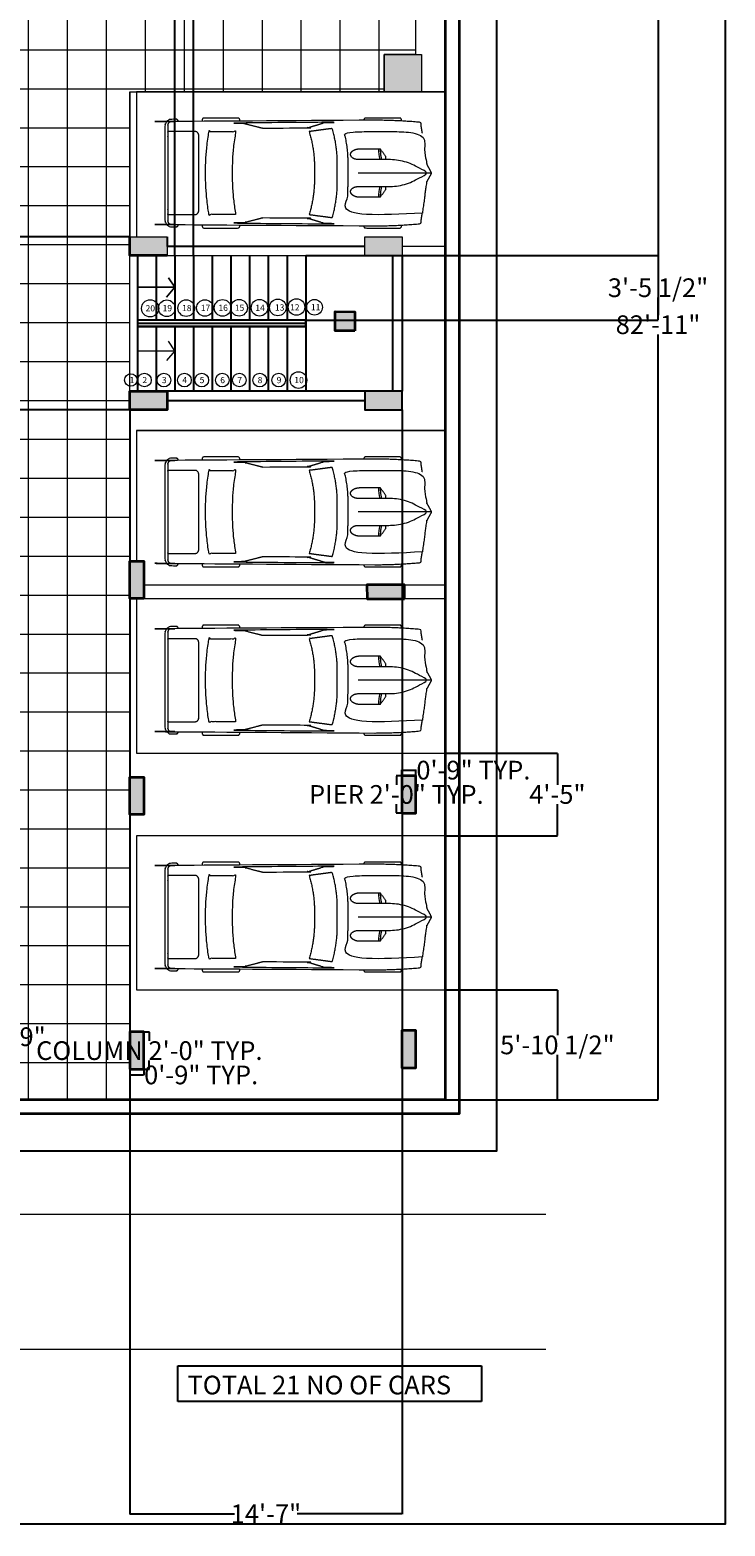
# Model space of a CAD drawing. Units: inches. Extents: x 48986 to 50522, y 132527 to 134098.
# Tile 3 of 4: x 50076 to 50522, y 132527 to 133488. Entities that reach past the tile are written whole.
import ezdxf

# ---------------------------------------------------------------- set-up
doc = ezdxf.new("R2010")
doc.units = ezdxf.units.IN
doc.header["$MEASUREMENT"] = 0
for name, color, linetype, lineweight in [('A-ANNO-DIMS', 2, 'Continuous', 18), ('A-ANNO-SYMB', 50, 'Continuous', 13), ('A-ANNO-TEXT', 7, 'Continuous', 18), ('A-ANNO-TTLB', 7, 'Continuous', 25), ('A-COLS-PATT', 215, 'Continuous', 13), ('A-EQPM-VEHC', 8, 'Continuous', 13), ('A-FLOR-PATT', 94, 'Continuous', 9), ('A-FLOR-PKNG', 140, 'Continuous', 18), ('C-PROP', 160, 'Continuous', 25), ('C-ROAD', 7, 'Continuous', 18), ('COLUMNS', 211, 'Continuous', 35), ('STAIRS', 10, 'Continuous', 25), ('WALLS', 140, 'Continuous', 35)]:
    doc.layers.add(name, color=color, linetype=linetype, lineweight=lineweight)
doc.styles.get("Standard").update_dxf_attribs({"font": 'arial.ttf'})
doc.dimstyles.get("Standard").update_dxf_attribs({"dimtxt": 12, "dimasz": 0.18, "dimexe": 0.18, "dimexo": 0.0625, "dimgap": 0.09, "dimtad": 0, "dimtih": 1, "dimtoh": 1, "dimdec": 1, "dimzin": 0, "dimdsep": 46, "dimlunit": 3, "dimtxsty": 'Standard', "dimcen": 0.09, "dimadec": 0, "dimazin": 0, "dimtfac": 1, "dimtdec": 1, "dimtofl": 0, "dimtmove": 0, "dimatfit": 3, "dimfxl": 1, "dimtolj": 1, "dimtzin": 0, "dimarcsym": 0})

# ---------------------------------------------------------------- blocks, each defined once
blk = doc.blocks.new('CAR-SEDAN-PLAN')
for p, q in [((35.28, 177.53), (35.28, 130.65)), ((25.73, 8.37), (44.83, 8.37))]:
    blk.add_line(p, q)
for centre, major_axis, start_param, end_param in [((19.85, 164.65), (-24.87, 0), 1.564964, 1.848039), ((50.71, 164.65), (24.87, 0), 4.435146, 4.718221)]:
    blk.add_ellipse(centre, major_axis=major_axis, ratio=0.842304, start_param=start_param, end_param=end_param)
for points, weights, knots in [([(60.93, 171.77), (56.4, 172.48), (51.85, 173.06), (46.33, 173.7), (40.84, 174.57), (38.25, 176), (35.65, 177.44), (35.28, 177.64), (34.91, 177.44), (32.32, 176), (29.72, 174.57), (24.24, 173.7), (18.71, 173.06), (14.16, 172.48), (9.64, 171.77), (7.88, 146.82), (9.23, 121.85), (17.23, 123.66), (25.51, 124.08), (35.28, 124.08), (45.06, 124.08), (53.33, 123.66), (61.34, 121.85), (62.69, 146.82), (60.93, 171.77)], [1, 0.999861960732, 1, 0.999699858145, 1, 1, 1, 0.835952709181, 1, 1, 1, 0.999699858145, 1, 0.999861960732, 1, 0.998625728423, 1, 0.994860280211, 1, 1, 1, 0.994860280211, 1, 0.998625728423, 1], [0, 0, 0, 0.033232, 0.033232, 0.082234, 0.082234, 1.082234, 1.082234, 2.244094, 2.244094, 3.244094, 3.244094, 3.293097, 3.293097, 3.326328, 3.326328, 3.431193, 3.431193, 3.634055, 3.634055, 4.634055, 4.634055, 4.836917, 4.836917, 4.941783, 4.941783, 4.941783]), ([(43.91, 145.56), (47.31, 144.74), (50.86, 144.76), (50.86, 138.04), (50.86, 131.32), (50.59, 126.02), (47.38, 125.71), (44.17, 125.4), (43.91, 130.65), (43.91, 140.58), (43.91, 150.52), (43.91, 163.57), (35.28, 174.41), (26.66, 163.57), (26.66, 150.52), (26.66, 140.58), (26.66, 130.65), (26.39, 125.4), (23.18, 125.71), (19.97, 126.02), (19.71, 131.32), (19.71, 138.04), (19.71, 144.76), (23.25, 144.74), (26.66, 145.56)], [1, 0.990000279832, 1, 1, 1, 0.735618766318, 1, 0.735618766318, 1, 1, 1, 0.956755789522, 1, 0.956755789522, 1, 1, 1, 0.735618766318, 1, 0.735618766318, 1, 1, 1, 0.990000279832, 1], [0, 0, 0, 0.283075, 0.283075, 1.283075, 1.283075, 2.771508, 2.771508, 4.259942, 4.259942, 5.259942, 5.259942, 5.85026, 5.85026, 6.440579, 6.440579, 7.440579, 7.440579, 8.929012, 8.929012, 10.417446, 10.417446, 11.417446, 11.417446, 11.700521, 11.700521, 11.700521]), ([(9.64, 171.77), (6.18, 171.25), (2.75, 170.65), (1.43, 155.99), (1.38, 141.3)], [1, 0.999923835344, 1, 0.999337806115, 1], [0, 0, 0, 0.02468451, 0.02468451, 0.0974728, 0.0974728, 0.0974728]), ([(69.18, 141.3), (69.13, 155.99), (67.82, 170.65), (64.38, 171.25), (60.93, 171.77)], [1, 0.999337806115, 1, 0.999923835344, 1], [0, 0, 0, 0.07278829, 0.07278829, 0.0974728, 0.0974728, 0.0974728]), ([(1.87, 158.39), (1.61, 158.39), (1.35, 158.39), (0.79, 158.39), (0.4, 158.06), (0, 157.72), (0, 157.26), (0, 146.28), (0, 135.3), (0, 134.83), (0.4, 134.5), (0.79, 134.17), (1.35, 134.17), (1.35, 134.17), (1.36, 134.17)], [1, 1, 1, 0.923879532511, 1, 0.923879532511, 1, 1, 1, 0.923879532511, 1, 0.923879532511, 1, 1, 1], [0, 0, 0, 1, 1, 1.785398, 1.785398, 2.570796, 2.570796, 3.570796, 3.570796, 4.356194, 4.356194, 5.141593, 5.141593, 6.141593, 6.141593, 6.141593]), ([(69.2, 134.17), (69.21, 134.17), (69.22, 134.17), (69.77, 134.17), (70.17, 134.5), (70.56, 134.83), (70.56, 135.3), (70.56, 146.28), (70.56, 157.26), (70.56, 157.72), (70.17, 158.06), (69.77, 158.39), (69.22, 158.39), (68.96, 158.39), (68.7, 158.39)], [1, 1, 1, 0.923879532511, 1, 0.923879532511, 1, 1, 1, 0.923879532511, 1, 0.923879532511, 1, 1, 1], [0, 0, 0, 1, 1, 1.785398, 1.785398, 2.570796, 2.570796, 3.570796, 3.570796, 4.356194, 4.356194, 5.141593, 5.141593, 6.141593, 6.141593, 6.141593]), ([(26.66, 148.39), (25.91, 148.39), (25.16, 148.39), (24.92, 148.39), (24.74, 148.26), (22.22, 146.51), (19.71, 144.76)], [1, 1, 1, 0.940892222322, 1, 1, 1], [0, 0, 0, 1, 1, 1.691083, 1.691083, 2.691083, 2.691083, 2.691083]), ([(50.86, 144.76), (48.34, 146.51), (45.83, 148.26), (45.64, 148.39), (45.4, 148.39), (44.65, 148.39), (43.91, 148.39)], [1, 1, 1, 0.940892222322, 1, 1, 1], [0, 0, 0, 1, 1, 1.691083, 1.691083, 2.691083, 2.691083, 2.691083]), ([(1.38, 141.68), (1.17, 76.13), (2.21, 10.6), (2.24, 8.37), (4.89, 8.37), (35.28, 8.37), (65.67, 8.37), (68.32, 8.37), (68.36, 10.6), (69.4, 76.13), (69.18, 141.68)], [1, 0.999967219517, 1, 0.711827418646, 1, 1, 1, 0.711827418646, 1, 0.999967219517, 1], [0, 0, 0, 0.016194, 0.016194, 1.573593, 1.573593, 2.573593, 2.573593, 4.130993, 4.130993, 4.147187, 4.147187, 4.147187]), ([(6.45, 69.32), (4.72, 62.5), (2.98, 55.69), (2.73, 82.7), (2.7, 109.71), (4.53, 103.71), (6.37, 97.71), (6.33, 83.51), (6.45, 69.32)], [1, 1, 1, 0.999994429546, 1, 1, 1, 0.999987377106, 1], [0, 0, 0, 1, 1, 1.006676, 1.006676, 2.006676, 2.006676, 2.016725, 2.016725, 2.016725]), ([(61.91, 99.15), (52.72, 101.89), (42.99, 102.47), (35.28, 102.47), (27.57, 102.47), (17.85, 101.89), (8.66, 99.15), (7.66, 106.57), (6.67, 114), (15.95, 116.64), (25.73, 117.16), (35.28, 117.16), (44.83, 117.16), (54.61, 116.64), (63.89, 114), (62.9, 106.57), (61.91, 99.15)], [1, 0.991000078903, 1, 1, 1, 0.991000078903, 1, 1, 1, 0.991394232237, 1, 1, 1, 0.991394232237, 1, 1, 1], [0, 0, 0, 0.268529, 0.268529, 1.268529, 1.268529, 1.537057, 1.537057, 2.537057, 2.537057, 2.799631, 2.799631, 3.799631, 3.799631, 4.062205, 4.062205, 5.062205, 5.062205, 5.062205]), ([(64.11, 69.32), (64.24, 83.51), (64.2, 97.71), (66.03, 103.71), (67.87, 109.71), (67.83, 82.7), (67.58, 55.69), (65.85, 62.5), (64.11, 69.32)], [1, 0.999987377106, 1, 1, 1, 0.999994429546, 1, 1, 1], [0, 0, 0, 0.010049, 0.010049, 1.010049, 1.010049, 1.016725, 1.016725, 2.016725, 2.016725, 2.016725]), ([(1.65, 54.65), (1.5, 54.65), (1.35, 54.65), (0, 54.65), (0, 53.52), (0, 42.54), (0, 31.57), (0, 30.44), (1.35, 30.44), (1.63, 30.44), (1.92, 30.44)], [1, 1, 1, 0.707106781187, 1, 1, 1, 0.707106781187, 1, 1, 1], [0, 0, 0, 1, 1, 2.570796, 2.570796, 3.570796, 3.570796, 5.141593, 5.141593, 6.141593, 6.141593, 6.141593]), ([(61.91, 51.96), (35.28, 47.39), (8.66, 51.96), (8.66, 43.42), (8.66, 34.88), (35.28, 30.31), (61.91, 34.88), (61.91, 43.42), (61.91, 51.96)], [1, 0.979868494456, 1, 1, 1, 0.979868494456, 1, 1, 1], [0, 0, 0, 0.401989, 0.401989, 1.401989, 1.401989, 1.803978, 1.803978, 2.803978, 2.803978, 2.803978]), ([(68.64, 30.44), (68.93, 30.44), (69.22, 30.44), (69.77, 30.44), (70.17, 30.77), (70.56, 31.1), (70.56, 31.57), (70.56, 42.54), (70.56, 53.52), (70.56, 53.99), (70.17, 54.32), (69.77, 54.65), (69.22, 54.65), (69.07, 54.65), (68.91, 54.65)], [1, 1, 1, 0.923879532511, 1, 0.923879532511, 1, 1, 1, 0.923879532511, 1, 0.923879532511, 1, 1, 1], [0, 0, 0, 1, 1, 1.785398, 1.785398, 2.570796, 2.570796, 3.570796, 3.570796, 4.356194, 4.356194, 5.141593, 5.141593, 6.141593, 6.141593, 6.141593]), ([(61.91, 8.37), (61.91, 17.2), (61.91, 26.03), (61.91, 28.29), (59.22, 28.29), (35.28, 28.29), (11.34, 28.29), (8.66, 28.29), (8.66, 26.03), (8.66, 17.2), (8.66, 8.37)], [1, 1, 1, 0.707106781187, 1, 1, 1, 0.707106781187, 1, 1, 1], [0, 0, 0, 1, 1, 2.570796, 2.570796, 3.570796, 3.570796, 5.141593, 5.141593, 6.141593, 6.141593, 6.141593]), ([(2.14, 15.28), (0.74, 14.89), (0.76, 13.65), (0.78, 12.11), (0.81, 10.58), (0.87, 6.62), (5.56, 6.62), (35.28, 6.62), (65, 6.62), (69.7, 6.62), (69.76, 10.58), (69.78, 12.11), (69.81, 13.65), (69.83, 14.89), (68.43, 15.28)], [1, 0.807168985933, 1, 0.999999981995, 1, 0.711827418646, 1, 1, 1, 0.711827418646, 1, 0.999999981995, 1, 0.807168985459, 1], [0, 0, 0, 1.262912, 1.262912, 1.263291, 1.263291, 2.82069, 2.82069, 3.82069, 3.82069, 5.37809, 5.37809, 5.378469, 5.378469, 6.641381, 6.641381, 6.641381])]:
    blk.add_rational_spline(points, weights, degree=2, knots=knots)
blk = doc.blocks.new('PARKING-STALL-99X198')
blk.add_lwpolyline([(198, 0), (198, 99), (0, 99), (0, 0)], close=True)
blk = doc.blocks.new('PIER-9X24-PERIM')
blk.add_lwpolyline([(9, 12), (9, 24), (0, 24), (0, 0), (9, 0), (9, 24)])
blk = doc.blocks.new('COL-9X24')
blk.add_lwpolyline([(0, 0), (9, 0), (9, 24), (0, 24)], close=True)
blk = doc.blocks.new('*D19')
at = {"layer": 'A-ANNO-DIMS', "color": 0, "lineweight": -2, "transparency": 16777216}
for p, q in [((50314.54, 133009.06), (50310.82, 133009.06)), ((50311, 133008.88), (50311, 133003.27)), ((50311, 132985.24), (50311, 132990.84)), ((50314.54, 132985.06), (50310.82, 132985.06))]:
    blk.add_line(p, q, dxfattribs=at)
at = {"layer": 'A-ANNO-DIMS', "color": 0, "transparency": 16777216}
for points in [[(50310.97, 133008.88), (50311.03, 133008.88), (50311, 133009.06)], [(50310.97, 132985.24), (50311.03, 132985.24), (50311, 132985.06)]]:
    blk.add_solid(points, dxfattribs=at)
at = {"layer": 'Defpoints', "color": 0, "transparency": 16777216}
for p in [(50311, 133009.06), (50314.6, 133009.06), (50314.6, 132985.06)]:
    blk.add_point(p, dxfattribs=at)
at = {"layer": 'A-ANNO-DIMS', "color": 0, "transparency": 16777216, "insert": (50311, 132997.06), "char_height": 12, "attachment_point": 5}
blk.add_mtext('\\A1;PIER 2\'-0" TYP.', dxfattribs=at)
blk = doc.blocks.new('*D20')
at = {"layer": 'A-ANNO-DIMS', "color": 0, "lineweight": -2, "transparency": 16777216}
for p, q in [((50314.6, 133009.12), (50314.6, 133012.84)), ((50314.78, 133012.66), (50323.42, 133012.66)), ((50323.6, 133009.12), (50323.6, 133012.84)), ((50323.6, 133012.66), (50323.78, 133012.66))]:
    blk.add_line(p, q, dxfattribs=at)
at = {"layer": 'A-ANNO-DIMS', "color": 0, "transparency": 16777216}
for points in [[(50314.78, 133012.69), (50314.78, 133012.63), (50314.6, 133012.66)], [(50323.42, 133012.69), (50323.42, 133012.63), (50323.6, 133012.66)]]:
    blk.add_solid(points, dxfattribs=at)
at = {"layer": 'Defpoints', "color": 0, "transparency": 16777216}
for p in [(50323.6, 133012.66), (50314.6, 133009.06), (50323.6, 133009.06)]:
    blk.add_point(p, dxfattribs=at)
at = {"layer": 'A-ANNO-DIMS', "color": 0, "transparency": 16777216, "insert": (50360.44, 133012.66), "char_height": 12, "attachment_point": 5}
blk.add_mtext('\\A1;0\'-9" TYP.', dxfattribs=at)
blk = doc.blocks.new('*D23')
at = {"layer": 'A-ANNO-DIMS', "color": 0, "lineweight": -2, "transparency": 16777216}
for p, q in [((50148.94, 132844.64), (50152.66, 132844.64)), ((50152.48, 132844.46), (50152.48, 132838.94)), ((50148.94, 132820.64), (50152.66, 132820.64)), ((50152.48, 132820.82), (50152.48, 132826.34))]:
    blk.add_line(p, q, dxfattribs=at)
at = {"layer": 'A-ANNO-DIMS', "color": 0, "transparency": 16777216}
for points in [[(50152.45, 132844.46), (50152.51, 132844.46), (50152.48, 132844.64)], [(50152.45, 132820.82), (50152.51, 132820.82), (50152.48, 132820.64)]]:
    blk.add_solid(points, dxfattribs=at)
at = {"layer": 'Defpoints', "color": 0, "transparency": 16777216}
for p in [(50148.88, 132844.64), (50152.48, 132844.64), (50148.88, 132820.64)]:
    blk.add_point(p, dxfattribs=at)
at = {"layer": 'A-ANNO-DIMS', "color": 0, "transparency": 16777216, "insert": (50152.48, 132832.64), "char_height": 12, "attachment_point": 5}
blk.add_mtext('\\A1;COLUMN 2\'-0" TYP.', dxfattribs=at)
blk = doc.blocks.new('*D24')
at = {"layer": 'A-ANNO-DIMS', "color": 0, "lineweight": -2, "transparency": 16777216}
for p, q in [((50139.88, 132820.58), (50139.88, 132816.86)), ((50140.06, 132817.04), (50148.7, 132817.04)), ((50148.88, 132820.58), (50148.88, 132816.86)), ((50148.88, 132817.04), (50149.06, 132817.04))]:
    blk.add_line(p, q, dxfattribs=at)
at = {"layer": 'A-ANNO-DIMS', "color": 0, "transparency": 16777216}
for points in [[(50140.06, 132817.07), (50140.06, 132817.01), (50139.88, 132817.04)], [(50148.7, 132817.07), (50148.7, 132817.01), (50148.88, 132817.04)]]:
    blk.add_solid(points, dxfattribs=at)
at = {"layer": 'Defpoints', "color": 0, "transparency": 16777216}
for p in [(50139.88, 132820.64), (50148.88, 132820.64), (50148.88, 132817.04)]:
    blk.add_point(p, dxfattribs=at)
at = {"layer": 'A-ANNO-DIMS', "color": 0, "transparency": 16777216, "insert": (50185.73, 132817.04), "char_height": 12, "attachment_point": 5}
blk.add_mtext('\\A1;0\'-9" TYP.', dxfattribs=at)
blk = doc.blocks.new('*D26')
at = {"layer": 'A-ANNO-DIMS', "color": 0, "lineweight": -2, "transparency": 16777216}
for p, q in [((50342.35, 133796.06), (50479.12, 133796.06)), ((50478.94, 133795.88), (50478.94, 133304.77)), ((50478.94, 132801.24), (50478.94, 133292.34)), ((50342.35, 132801.06), (50479.12, 132801.06))]:
    blk.add_line(p, q, dxfattribs=at)
at = {"layer": 'A-ANNO-DIMS', "color": 0, "transparency": 16777216}
for points in [[(50478.91, 133795.88), (50478.97, 133795.88), (50478.94, 133796.06)], [(50478.91, 132801.24), (50478.97, 132801.24), (50478.94, 132801.06)]]:
    blk.add_solid(points, dxfattribs=at)
at = {"layer": 'Defpoints', "color": 0, "transparency": 16777216}
for p in [(50342.29, 133796.06), (50342.29, 132801.06), (50478.94, 132801.06)]:
    blk.add_point(p, dxfattribs=at)
at = {"layer": 'A-ANNO-DIMS', "color": 0, "transparency": 16777216, "insert": (50478.94, 133298.56), "char_height": 12, "attachment_point": 5}
blk.add_mtext('\\A1;82\'-11"', dxfattribs=at)
blk = doc.blocks.new('*D29')
at = {"layer": 'A-ANNO-DIMS', "color": 0, "lineweight": -2, "transparency": 16777216}
for p, q in [((50342.35, 132871.56), (50414.52, 132871.56)), ((50414.34, 132871.38), (50414.34, 132842.6)), ((50414.34, 132801.24), (50414.34, 132830.01)), ((50342.35, 132801.06), (50414.52, 132801.06))]:
    blk.add_line(p, q, dxfattribs=at)
at = {"layer": 'A-ANNO-DIMS', "color": 0, "transparency": 16777216}
for points in [[(50414.31, 132871.38), (50414.37, 132871.38), (50414.34, 132871.56)], [(50414.31, 132801.24), (50414.37, 132801.24), (50414.34, 132801.06)]]:
    blk.add_solid(points, dxfattribs=at)
at = {"layer": 'Defpoints', "color": 0, "transparency": 16777216}
for p in [(50342.29, 132871.56), (50342.29, 132801.06), (50414.34, 132801.06)]:
    blk.add_point(p, dxfattribs=at)
at = {"layer": 'A-ANNO-DIMS', "color": 0, "transparency": 16777216, "insert": (50414.34, 132836.31), "char_height": 12, "attachment_point": 5}
blk.add_mtext('\\A1;5\'-10 1/2"', dxfattribs=at)
blk = doc.blocks.new('*D30')
at = {"layer": 'A-ANNO-DIMS', "color": 0, "lineweight": -2, "transparency": 16777216}
for p, q in [((50139.82, 133355.06), (49029.36, 133355.06)), ((49029.54, 133354.88), (49029.54, 133305.73)), ((49029.54, 133244.15), (49029.54, 133293.29)), ((50139.82, 133243.97), (49029.36, 133243.97))]:
    blk.add_line(p, q, dxfattribs=at)
at = {"layer": 'A-ANNO-DIMS', "color": 0, "transparency": 16777216}
for points in [[(49029.51, 133354.88), (49029.57, 133354.88), (49029.54, 133355.06)], [(49029.51, 133244.15), (49029.57, 133244.15), (49029.54, 133243.97)]]:
    blk.add_solid(points, dxfattribs=at)
at = {"layer": 'Defpoints', "color": 0, "transparency": 16777216}
for p in [(49029.54, 133355.06), (50139.88, 133355.06), (50139.88, 133243.97)]:
    blk.add_point(p, dxfattribs=at)
at = {"layer": 'A-ANNO-DIMS', "color": 0, "transparency": 16777216, "insert": (49029.54, 133299.51), "char_height": 12, "attachment_point": 5}
blk.add_mtext('\\A1;9\'-3"', dxfattribs=at)
blk = doc.blocks.new('*D31')
at = {"layer": 'A-ANNO-DIMS', "color": 0, "lineweight": -2, "transparency": 16777216}
for p, q in [((50139.88, 133243.91), (50139.88, 132535.17)), ((50314.72, 133243.91), (50314.72, 132535.17)), ((50140.06, 132535.35), (50207.17, 132535.35)), ((50314.54, 132535.35), (50247.44, 132535.35))]:
    blk.add_line(p, q, dxfattribs=at)
at = {"layer": 'A-ANNO-DIMS', "color": 0, "transparency": 16777216}
for points in [[(50140.06, 132535.38), (50140.06, 132535.32), (50139.88, 132535.35)], [(50314.54, 132535.38), (50314.54, 132535.32), (50314.72, 132535.35)]]:
    blk.add_solid(points, dxfattribs=at)
at = {"layer": 'Defpoints', "color": 0, "transparency": 16777216}
for p in [(50139.88, 133243.97), (50314.72, 133243.97), (50314.72, 132535.35)]:
    blk.add_point(p, dxfattribs=at)
at = {"layer": 'A-ANNO-DIMS', "color": 0, "transparency": 16777216, "insert": (50227.3, 132535.35), "char_height": 12, "attachment_point": 5}
blk.add_mtext('\\A1;14\'-7"', dxfattribs=at)
blk = doc.blocks.new('*D37')
at = {"layer": 'A-ANNO-DIMS', "color": 0, "lineweight": -2, "transparency": 16777216}
for p, q in [((50342.35, 133023.56), (50414.52, 133023.56)), ((50414.34, 133023.38), (50414.34, 133003.25)), ((50414.34, 132970.74), (50414.34, 132990.86)), ((50342.35, 132970.56), (50414.52, 132970.56))]:
    blk.add_line(p, q, dxfattribs=at)
at = {"layer": 'A-ANNO-DIMS', "color": 0, "transparency": 16777216}
for points in [[(50414.31, 133023.38), (50414.37, 133023.38), (50414.34, 133023.56)], [(50414.31, 132970.74), (50414.37, 132970.74), (50414.34, 132970.56)]]:
    blk.add_solid(points, dxfattribs=at)
at = {"layer": 'Defpoints', "color": 0, "transparency": 16777216}
for p in [(50342.29, 133023.56), (50342.29, 132970.56), (50414.34, 132970.56)]:
    blk.add_point(p, dxfattribs=at)
at = {"layer": 'A-ANNO-DIMS', "color": 0, "transparency": 16777216, "insert": (50414.34, 132997.06), "char_height": 12, "attachment_point": 5}
blk.add_mtext('\\A1;4\'-5"', dxfattribs=at)
blk = doc.blocks.new('*D38')
at = {"layer": 'A-ANNO-DIMS', "color": 0, "lineweight": -2, "transparency": 16777216}
for p, q in [((49995.94, 132882.05), (50068.11, 132882.05)), ((50067.93, 132881.87), (50067.93, 132847.77)), ((50067.93, 132801.24), (50067.93, 132835.33)), ((49995.94, 132801.06), (50068.11, 132801.06))]:
    blk.add_line(p, q, dxfattribs=at)
at = {"layer": 'A-ANNO-DIMS', "color": 0, "transparency": 16777216}
for points in [[(50067.9, 132881.87), (50067.96, 132881.87), (50067.93, 132882.05)], [(50067.9, 132801.24), (50067.96, 132801.24), (50067.93, 132801.06)]]:
    blk.add_solid(points, dxfattribs=at)
at = {"layer": 'Defpoints', "color": 0, "transparency": 16777216}
for p in [(49995.88, 132882.05), (49995.88, 132801.06), (50067.93, 132801.06)]:
    blk.add_point(p, dxfattribs=at)
at = {"layer": 'A-ANNO-DIMS', "color": 0, "transparency": 16777216, "insert": (50067.93, 132841.55), "char_height": 12, "attachment_point": 5}
blk.add_mtext('\\A1;6\'-9"', dxfattribs=at)
blk = doc.blocks.new('*D42')
at = {"layer": 'A-ANNO-DIMS', "color": 0, "lineweight": -2, "transparency": 16777216}
for p, q in [((50168.85, 133343.12), (50168.85, 133901.29)), ((50169.03, 133901.11), (50180.67, 133901.11)), ((50180.85, 133343.12), (50180.85, 133901.29)), ((50180.85, 133901.11), (50181.03, 133901.11))]:
    blk.add_line(p, q, dxfattribs=at)
at = {"layer": 'A-ANNO-DIMS', "color": 0, "transparency": 16777216}
for points in [[(50169.03, 133901.14), (50169.03, 133901.08), (50168.85, 133901.11)], [(50180.67, 133901.14), (50180.67, 133901.08), (50180.85, 133901.11)]]:
    blk.add_solid(points, dxfattribs=at)
at = {"layer": 'Defpoints', "color": 0, "transparency": 16777216}
for p in [(50180.85, 133901.11), (50168.85, 133343.06), (50180.85, 133343.06)]:
    blk.add_point(p, dxfattribs=at)
at = {"layer": 'A-ANNO-DIMS', "color": 0, "transparency": 16777216, "insert": (50196.51, 133901.11), "char_height": 12, "attachment_point": 5}
blk.add_mtext('\\A1;1\'-0"', dxfattribs=at)
blk = doc.blocks.new('*D43')
at = {"layer": 'A-ANNO-DIMS', "color": 0, "lineweight": -2, "transparency": 16777216}
for p, q in [((50252.91, 133343.06), (50479.12, 133343.06)), ((50478.94, 133342.88), (50478.94, 133328.58)), ((50478.94, 133301.69), (50478.94, 133315.99)), ((50252.91, 133301.51), (50479.12, 133301.51))]:
    blk.add_line(p, q, dxfattribs=at)
at = {"layer": 'A-ANNO-DIMS', "color": 0, "transparency": 16777216}
for points in [[(50478.91, 133342.88), (50478.97, 133342.88), (50478.94, 133343.06)], [(50478.91, 133301.69), (50478.97, 133301.69), (50478.94, 133301.51)]]:
    blk.add_solid(points, dxfattribs=at)
at = {"layer": 'Defpoints', "color": 0, "transparency": 16777216}
for p in [(50252.85, 133343.06), (50252.85, 133301.51), (50478.94, 133301.51)]:
    blk.add_point(p, dxfattribs=at)
at = {"layer": 'A-ANNO-DIMS', "color": 0, "transparency": 16777216, "insert": (50478.94, 133322.29), "char_height": 12, "attachment_point": 5}
blk.add_mtext('\\A1;3\'-5 1/2"', dxfattribs=at)

msp = doc.modelspace()

# ---------------------------------------------------------------- hatches: boundary and pattern name
at = {"layer": 'A-COLS-PATT'}
h = msp.add_hatch(color=256, dxfattribs=at)
h.dxf.hatch_style = 1
h.paths.add_polyline_path([(50327.12, 133472.06), (50303.12, 133472.06), (50303.12, 133448.06), (50327.12, 133448.06)])
h.paths.add_polyline_path([(50163.88, 133355.06), (50151.88, 133355.06), (50139.88, 133355.06), (50139.88, 133343.06), (50163.88, 133343.06)])
h.paths.add_polyline_path([(50314.72, 133355.06), (50302.72, 133355.06), (50290.72, 133355.06), (50290.72, 133343.06), (50314.72, 133343.06)])
h.paths.add_polyline_path([(50163.88, 133255.97), (50151.88, 133255.97), (50139.88, 133255.97), (50139.88, 133243.97), (50163.88, 133243.97)])
h.paths.add_polyline_path([(50314.72, 133255.97), (50302.72, 133255.97), (50290.72, 133255.97), (50290.72, 133243.97), (50314.72, 133243.97)])
h.paths.add_polyline_path([(50148.88, 133146.77), (50139.88, 133146.77), (50139.88, 133122.77), (50148.88, 133122.77)])
h.paths.add_polyline_path([(50316.2, 133131.56), (50292.12, 133131.56), (50292.2, 133122.56), (50316.2, 133122.56)])
h.paths.add_polyline_path([(50148.88, 133008.11), (50139.88, 133008.11), (50139.88, 132984.11), (50148.88, 132984.11)])
h.paths.add_polyline_path([(50323.6, 133009.06), (50314.6, 133009.06), (50314.6, 132985.06), (50323.6, 132985.06)])
h.paths.add_polyline_path([(50148.88, 132844.64), (50139.88, 132844.64), (50139.88, 132820.64), (50148.88, 132820.64)])
h.paths.add_polyline_path([(50323.6, 132845.59), (50314.6, 132845.59), (50314.6, 132821.59), (50323.6, 132821.59)])
h = msp.add_hatch(color=256, dxfattribs=at)
h.dxf.hatch_style = 1
h.paths.add_polyline_path([(50284.45, 133306.79), (50271.77, 133306.98), (50271.77, 133294.68), (50284.45, 133294.68)])
at = {"layer": 'A-FLOR-PATT'}
h = msp.add_hatch(dxfattribs=at)
h.set_pattern_fill('NET', color=256, scale=200)
h.paths.add_polyline_path([(50323.33, 133597.94), (50298.79, 133598.06), (50199.79, 133598.06), (49957.56, 133598.06), (49597.63, 133598.06), (49221.79, 133598.06), (49221.79, 132801.06), (49253.29, 132801.06), (49253.29, 132832.63), (49251.14, 132832.63), (49251.14, 132842.53), (49253.29, 132842.53), (49253.29, 132956.08), (49251.14, 132956.08), (49251.14, 132965.97), (49253.29, 132965.97), (49253.29, 133105.3), (49251.14, 133105.3), (49251.14, 133115.2), (49253.29, 133115.2), (49253.29, 133143.75), (49253.29, 133153.65), (49253.29, 133244.43), (49251.14, 133244.43), (49251.14, 133254.33), (49253.29, 133254.33), (49253.29, 133283.54), (49253.29, 133293.44), (49253.29, 133335.08), (49251.14, 133335.08), (49248.66, 133335.08), (49248.66, 133344.97), (49251.14, 133344.97), (49253.29, 133344.97), (49253.29, 133387.65), (49253.29, 133397.55), (49253.29, 133425.06), (49253.29, 133426.99), (49420.79, 133426.99), (49423.36, 133426.99), (49423.36, 133344.97), (49425.09, 133344.97), (49425.09, 133335.08), (49423.36, 133335.08), (49423.36, 132813.06), (49567.36, 132813.06), (49567.36, 133229.31), (49567.36, 133241.64), (49567.36, 133265.64), (49567.36, 133335.08), (49567.36, 133344.97), (49567.36, 133361.98), (49567.36, 133385.98), (49567.36, 133426.99), (49591.36, 133426.99), (49690.36, 133426.99), (49817.62, 133426.99), (49817.62, 133427.11), (49841.62, 133427.11), (49995.88, 133426.99), (49995.88, 132801.06), (50139.88, 132801.06), (50139.88, 133259.08, -0.361241), (50136.6, 133263.03, -0.361241), (50139.88, 133266.99), (50139.88, 133448.06), (50303.12, 133448.06), (50303.12, 133472.06), (50323.33, 133472.06)])

# ---------------------------------------------------------------- linework, layer by layer
at = {"layer": 'A-ANNO-SYMB'}
msp.add_line((50168.85, 133281.79), (50163.46, 133275.48), dxfattribs=at)
msp.add_lwpolyline([(50168.85, 133322.6), (50144.85, 133322.6), (50144.85, 133322.6), (50168.85, 133322.6), (50163.46, 133316.29), (50168.85, 133322.6), (50164.69, 133328.74)], close=True, dxfattribs=at)
msp.add_lwpolyline([(50144.85, 133281.79), (50168.85, 133281.79), (50164.69, 133287.93)], dxfattribs=at)
for centre, radius in [((50152.98, 133309.06), 5.5), ((50163.68, 133309.13), 5.34), ((50176.16, 133309.21), 5.34), ((50188.17, 133309.31), 5.31), ((50199.52, 133309.36), 5.33), ((50210.05, 133309.43), 5.35), ((50223.19, 133309.43), 5.31), ((50234.97, 133309.64), 5.34), ((50246.93, 133309.91), 5.3), ((50258.5, 133309.76), 5.02), ((50140.62, 133263.03), 4.02), ((50149.35, 133263.03), 4.36), ((50161.84, 133263), 4.38), ((50175.03, 133263.04), 4.39), ((50186.12, 133263.01), 4.38), ((50199.32, 133263), 4.39), ((50210.29, 133263.04), 4.34), ((50223.32, 133263), 4.39), ((50235.5, 133263), 4.38), ((50248.22, 133263), 5.33)]:
    msp.add_circle(centre, radius, dxfattribs=at)
at = {"layer": 'A-ANNO-TTLB'}
for p, q in [((50170.76, 132607.4), (50170.76, 132630.42)), ((50170.76, 132630.42), (50181.49, 132630.42)), ((50176.98, 132630.42), (50365.55, 132630.42)), ((50365.55, 132630.42), (50365.55, 132607.4)), ((50365.55, 132607.4), (50170.76, 132607.4))]:
    msp.add_line(p, q, dxfattribs=at)
msp.add_lwpolyline([(48985.99, 134098.01), (50521.96, 134098.01), (50521.96, 132528.75), (48985.99, 132528.75)], close=True, dxfattribs=at)
at = {"layer": 'A-FLOR-PKNG'}
for p, q in [((50139.88, 133448.06), (50342.29, 133448.06)), ((50139.88, 133426.99), (50139.88, 133426.99)), ((50148.88, 133131.56), (50342.29, 133131.56))]:
    msp.add_line(p, q, dxfattribs=at)
for points in [[(50323.33, 133597.94), (50298.79, 133598.06), (50323.33, 133597.94), (50323.33, 133472.06), (50303.12, 133472.06), (50303.12, 133448.06), (50303.12, 133472.06), (50327.12, 133472.06), (50327.12, 133448.06)], [(50139.88, 132801.06), (50139.88, 133448.06), (50139.88, 133355.06), (50139.88, 133355.06), (50151.88, 133355.06), (50163.88, 133355.06), (50163.88, 133343.06), (50290.72, 133343.06), (50290.72, 133355.06), (50302.72, 133355.06), (50314.72, 133355.06), (50314.72, 133343.06)], [(50342.29, 133349.06), (50342.29, 133448.06), (50144.29, 133448.06), (50144.29, 133355.06)], [(50314.72, 133349.06), (50342.29, 133349.06), (50342.29, 133230.56), (50144.29, 133230.56), (50144.29, 133146.77)], [(50144.29, 133230.56), (50342.29, 133230.56), (50342.29, 133131.56), (50342.29, 133122.56), (50144.29, 133122.56), (50144.29, 133023.56), (50342.29, 133023.56), (50342.29, 132970.56), (50144.29, 132970.56)], [(50342.29, 133023.56), (50342.29, 133122.56), (50144.29, 133122.56)]]:
    msp.add_lwpolyline(points, dxfattribs=at)
at = {"layer": 'C-PROP'}
msp.add_lwpolyline([(49188.79, 133829.06), (50375.29, 133829.06), (50375.29, 132768.06), (49188.79, 132768.06)], close=True, dxfattribs=at)
at = {"layer": 'C-ROAD'}
for p, q in [((49101.59, 132727.74), (50406.89, 132727.74)), ((49101.59, 132641.08), (50406.89, 132641.08))]:
    msp.add_line(p, q, dxfattribs=at)
at = {"layer": 'COLUMNS'}
msp.add_lwpolyline([(50163.88, 133343.06), (50139.88, 133343.06), (50139.88, 133355.06)], dxfattribs=at)
for points in [[(50284.45, 133294.68), (50271.77, 133294.68), (50271.77, 133306.98), (50284.45, 133306.79)], [(50163.88, 133255.97), (50163.88, 133243.97), (50139.88, 133243.97), (50139.88, 133255.97), (50151.88, 133255.97)], [(50316.2, 133122.56), (50316.2, 133131.56), (50292.12, 133131.56), (50292.2, 133122.56)]]:
    msp.add_lwpolyline(points, close=True, dxfattribs=at)
at = {"layer": 'STAIRS'}
for p, q in [((50144.85, 133343.06), (50144.85, 133255.97)), ((50156.85, 133343.06), (50156.85, 133301.51)), ((50168.85, 133343.06), (50168.85, 133301.51)), ((50180.85, 133343.06), (50180.85, 133301.51)), ((50192.85, 133343.06), (50192.85, 133301.51)), ((50204.85, 133343.06), (50204.85, 133301.51)), ((50216.85, 133343.06), (50216.85, 133301.51)), ((50228.85, 133343.06), (50228.85, 133301.51)), ((50240.85, 133343.06), (50240.85, 133301.51)), ((50252.85, 133343.06), (50252.85, 133255.97)), ((50144.85, 133299.51), (50252.85, 133299.51)), ((50156.85, 133297.51), (50156.85, 133255.97)), ((50168.85, 133297.51), (50168.85, 133255.97)), ((50180.85, 133297.51), (50180.85, 133255.97)), ((50192.85, 133297.51), (50192.85, 133255.97)), ((50204.85, 133297.51), (50204.85, 133255.97)), ((50216.85, 133297.51), (50216.85, 133255.97)), ((50228.85, 133297.51), (50228.85, 133255.97)), ((50240.85, 133297.51), (50240.85, 133255.97)), ((50163.88, 133249.97), (50290.72, 133249.97))]:
    msp.add_line(p, q, dxfattribs=at)
for points in [[(50163.88, 133355.06), (50163.88, 133349.06), (50167.01, 133349.06), (50168.67, 133349.06), (50290.72, 133349.06)], [(50290.72, 133343.06), (50314.72, 133343.06), (50314.72, 133255.97), (50308.72, 133255.97), (50308.72, 133343.06)], [(50252.85, 133297.51), (50144.85, 133297.51), (50252.85, 133297.51), (50252.85, 133301.51), (50144.85, 133301.51), (50144.85, 133297.51)], [(50290.72, 133255.97), (50290.72, 133243.97), (50314.72, 133243.97), (50314.72, 133255.97), (50302.72, 133255.97), (50290.72, 133255.97), (50163.26, 133255.97)]]:
    msp.add_lwpolyline(points, dxfattribs=at)
at = {"layer": 'WALLS'}
msp.add_lwpolyline([(49212.79, 133805.06), (50351.29, 133805.06), (50351.29, 132792.06), (49212.79, 132792.06)], close=True, dxfattribs=at)
msp.add_lwpolyline([(50342.29, 133796.06), (50342.29, 132801.06), (49221.79, 132801.06), (49221.79, 133796.06), (50342.29, 133796.06), (50298.79, 133796.06), (50298.79, 133598.06), (50298.79, 133796.06), (50199.79, 133796.06), (50199.79, 133598.06), (50298.79, 133598.06), (49957.56, 133598.06), (49597.63, 133598.06), (49597.63, 133796.06), (49696.63, 133796.06), (49696.63, 133598.06), (49597.63, 133598.06), (49221.79, 133598.06), (49221.79, 133426.99)], dxfattribs=at)

# ---------------------------------------------------------------- block references
at = {"layer": 'A-EQPM-VEHC'}
for p, rotation in [((50155.91, 133431.18), 270.0000000000086), ((50155.91, 133213.68), 269.9999999999914), ((50155.91, 133105.68), 270.0000000000086), ((50155.91, 132953.68), 270.0000000000086)]:
    msp.add_blockref('CAR-SEDAN-PLAN', p, dxfattribs=dict(at, rotation=rotation))
at = {"layer": 'A-FLOR-PKNG', "rotation": 180}
msp.add_blockref('PARKING-STALL-99X198', (50342.29, 132970.56), dxfattribs=at)
at = {"layer": 'COLUMNS', "extrusion": (0, 0, -1), "zscale": -1}
for name, p in [('COL-9X24', (-50148.88, 133122.77)), ('PIER-9X24-PERIM', (-50148.88, 132984.11))]:
    msp.add_blockref(name, p, dxfattribs=at)
at = {"layer": 'COLUMNS'}
for name, p in [('PIER-9X24-PERIM', (50314.6, 132985.06)), ('COL-9X24', (50139.88, 132820.64)), ('PIER-9X24-PERIM', (50314.6, 132821.59))]:
    msp.add_blockref(name, p, dxfattribs=at)

# ---------------------------------------------------------------- texts
at = {"layer": 'A-ANNO-TEXT', "attachment_point": 1}
for s, width, insert, char_height in [('20', 5.3219, (50150.09, 133311.1), 4), ('19', 5.3219, (50161, 133311.17), 4), ('18', 5.3219, (50173.48, 133311.25), 4), ('17', 5.3219, (50185.49, 133311.32), 4), ('16', 5.3219, (50196.84, 133311.4), 4), ('15', 5.3219, (50207.35, 133311.47), 4), ('14', 5.3219, (50220.52, 133311.43), 4), ('13', 5.3219, (50233.1, 133311.62), 4), ('12', 5.3219, (50242.82, 133311.7), 4), ('11', 5.3219, (50256.21, 133311.77), 4), ('1', 5.3219, (50139.88, 133265.04), 4), ('2', 5.3219, (50148.03, 133265.04), 4), ('3', 5.3219, (50160.53, 133265.04), 4), ('4', 5.3219, (50173.65, 133265.04), 4), ('5', 5.3219, (50184.79, 133265.04), 4), ('6', 5.3219, (50198, 133265.04), 4), ('7', 5.3219, (50209, 133265.04), 4), ('8', 5.3219, (50222.01, 133265.04), 4), ('9', 5.3219, (50234.19, 133265.04), 4), ('10', 5.3219, (50245.55, 133265.04), 4), ('TOTAL 21 NO OF CARS', 227.0688, (50176.98, 132623.99), 12)]:
    msp.add_mtext_dynamic_manual_height_columns(s, width=width, gutter_width=1, heights=[0], dxfattribs=dict(at, insert=insert, char_height=char_height))

# ---------------------------------------------------------------- dimensions: what is measured, and where the dimension line sits
at = {"layer": 'A-ANNO-DIMS'}
for base, p1, p2, picture, middle in [((50180.85, 133901.11), (50168.85, 133343.06), (50180.85, 133343.06), '*D42', (50196.51, 133901.11)), ((50314.72, 132535.35), (50139.88, 133243.97), (50314.72, 133243.97), '*D31', (50227.3, 132535.35))]:
    dim = msp.add_linear_dim(base=base, p1=p1, p2=p2, dimstyle='Standard', override={"dimdec": 1, "dimlfac": 1, "dimrnd": 0, "dimzin": 1, "dimdsep": 46, "dimlunit": 4, "dimfrac": 2}, dxfattribs=at)
    dim.commit()
    dim.dimension.update_dxf_attribs({"geometry": picture, "text_midpoint": middle})
for base, p1, p2, angle, picture, middle in [((50478.94, 132801.06), (50342.29, 133796.06), (50342.29, 132801.06), 90, '*D26', (50478.94, 133298.56)), ((49029.54, 133355.06), (50139.88, 133243.97), (50139.88, 133355.06), 90, '*D30', (49029.54, 133299.51)), ((50478.943, 133301.5136), (50252.8512, 133343.0565), (50252.8512, 133301.5136), 90, '*D43', (50478.943, 133322.285)), ((50414.34, 132970.56), (50342.29, 133023.56), (50342.29, 132970.56), 270, '*D37', (50414.34, 132997.06)), ((50067.93, 132801.06), (49995.88, 132882.05), (49995.88, 132801.06), 270, '*D38', (50067.93, 132841.55)), ((50414.34, 132801.06), (50342.29, 132871.56), (50342.29, 132801.06), 270, '*D29', (50414.34, 132836.31))]:
    dim = msp.add_linear_dim(base=base, p1=p1, p2=p2, angle=angle, dimstyle='Standard', override={"dimdec": 1, "dimlfac": 1, "dimrnd": 0, "dimzin": 1, "dimdsep": 46, "dimlunit": 4, "dimfrac": 2}, dxfattribs=at)
    dim.commit()
    dim.dimension.update_dxf_attribs({"geometry": picture, "text_midpoint": middle})
for base, p1, p2, picture, middle in [((50323.6, 133012.66), (50314.6, 133009.06), (50323.6, 133009.06), '*D20', (50360.44, 133012.66)), ((50148.88, 132817.04), (50139.88, 132820.64), (50148.88, 132820.64), '*D24', (50185.73, 132817.04))]:
    dim = msp.add_linear_dim(base=base, p1=p1, p2=p2, text='<> TYP.', dimstyle='Standard', override={"dimdec": 1, "dimlfac": 1, "dimrnd": 0, "dimzin": 1, "dimdsep": 46, "dimlunit": 4, "dimfrac": 2}, dxfattribs=at)
    dim.commit()
    dim.dimension.update_dxf_attribs({"geometry": picture, "text_midpoint": middle})
for base, p1, p2, text, picture, middle in [((50311, 133009.06), (50314.6, 132985.06), (50314.6, 133009.06), 'PIER <> TYP.', '*D19', (50311, 132997.06)), ((50152.48, 132844.64), (50148.88, 132820.64), (50148.88, 132844.64), 'COLUMN <> TYP.', '*D23', (50152.48, 132832.64))]:
    dim = msp.add_linear_dim(base=base, p1=p1, p2=p2, angle=90, text=text, dimstyle='Standard', override={"dimdec": 1, "dimlfac": 1, "dimrnd": 0, "dimzin": 1, "dimdsep": 46, "dimlunit": 4, "dimfrac": 2}, dxfattribs=at)
    dim.commit()
    dim.dimension.update_dxf_attribs({"geometry": picture, "text_midpoint": middle})

doc.saveas('drawing.dxf')
